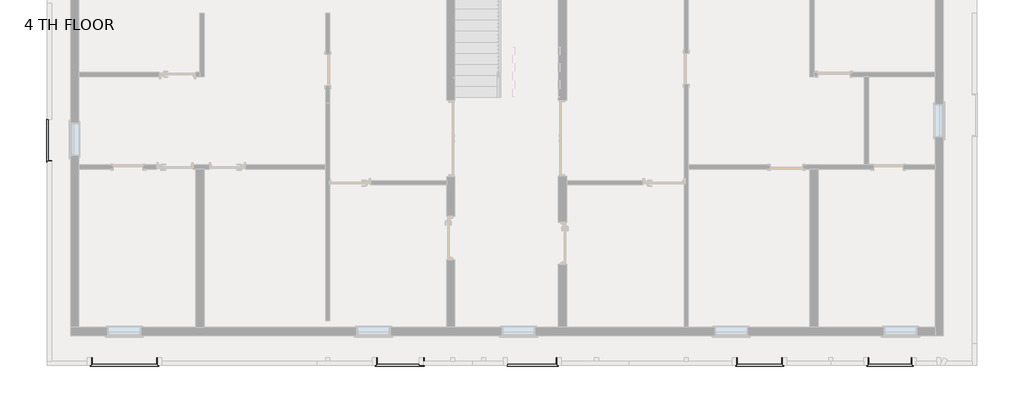
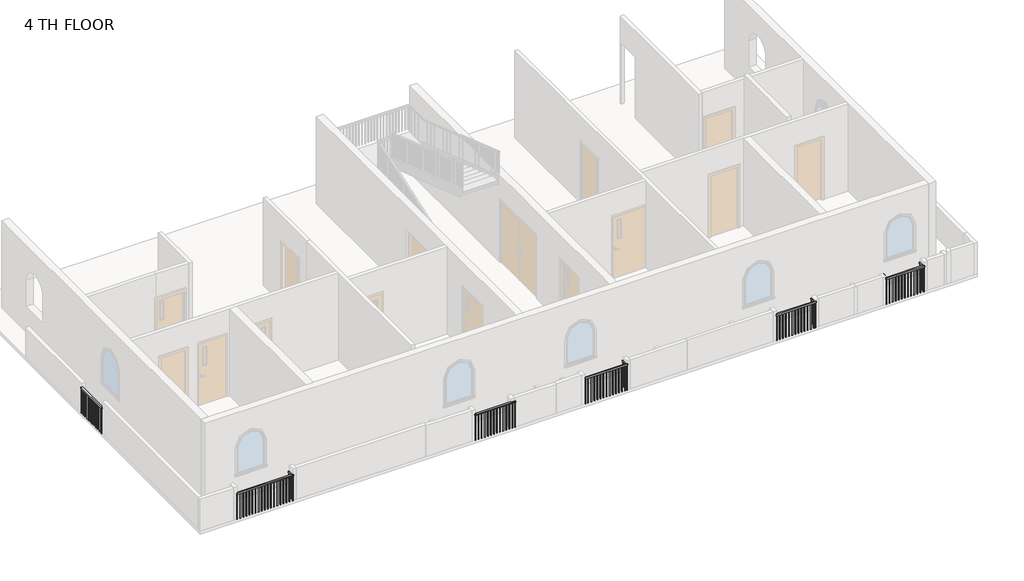
# One storey, part 3 of 7: 6 railings.
"""IFC4 building model written with IfcOpenShell, lengths in millimetres."""

from ifc_helpers import new_model, si_unit, frame, origin, place, context, project, spatial, polyline, outline, extrude, faceted_brep, element, save

model = new_model("IFC4")

# Units and contexts
model_context = context("Model", 3, world=origin())
ifc_project = project(units=[si_unit("LENGTHUNIT", "METRE", prefix="MILLI")], contexts=[model_context])

# Site, building, storey
site = spatial("IfcSite", under=ifc_project)
building = spatial("IfcBuilding", under=site)
storey = spatial("IfcBuildingStorey", under=building, Name="4 TH FLOOR", Elevation=12801.6)

# Railings
placement = place(None, origin())
element("IfcRailing", 1, ObjectType="Handrail - Rectangular", at=placement, inside=storey, context=model_context, shape_type="SolidModel", body=[
    faceted_brep([(-11856.9067989, -4623.6932193, 13716.0), (-11856.9067989, -4623.6932193, 13665.2), (-11907.7067989, -4623.6932193, 13665.2), (-11907.7067989, -4623.6932193, 13716.0), (-11856.9067989, -4801.4932661, 13716.0), (-11856.9067989, -4801.4932661, 13665.2), (-11907.7067989, -4852.2932661, 13665.2), (-11907.7067989, -4852.2932661, 13716.0), (-10071.3470335, -4801.4932661, 13716.0), (-10071.3470335, -4801.4932661, 13665.2), (-10020.5470335, -4852.2932661, 13665.2), (-10020.5470335, -4852.2932661, 13716.0), (-10071.3470335, -4623.6932193, 13716.0), (-10020.5470335, -4623.6932193, 13716.0), (-10020.5470335, -4623.6932193, 13665.2), (-10071.3470335, -4623.6932193, 13665.2)], [[[0, 1, 2, 3]], [[1, 0, 4, 5]], [[2, 1, 5, 6]], [[3, 2, 6, 7]], [[0, 3, 7, 4]], [[5, 4, 8, 9]], [[6, 5, 9, 10]], [[7, 6, 10, 11]], [[4, 7, 11, 8]], [[12, 13, 14, 15]], [[9, 8, 12, 15]], [[10, 9, 15, 14]], [[11, 10, 14, 13]], [[8, 11, 13, 12]]]),
    extrude(outline(polyline([(-10036.4220335, -4633.2182661), (-10055.4720335, -4633.2182661), (-10055.4720335, -4614.1682661), (-10036.4220335, -4614.1682661), (-10036.4220335, -4633.2182661)])), frame((0.0, 0.0, 12801.6), z_axis=(0.0, 0.0, 1.0), x_axis=(1.0, 0.0, 0.0)), (0.0, 0.0, 1.0), 863.6),
    extrude(outline(polyline([(-10036.4220335, -4734.8182661), (-10055.4720335, -4734.8182661), (-10055.4720335, -4715.7682661), (-10036.4220335, -4715.7682661), (-10036.4220335, -4734.8182661)])), frame((0.0, 0.0, 12801.6), z_axis=(0.0, 0.0, 1.0), x_axis=(1.0, 0.0, 0.0)), (0.0, 0.0, 1.0), 863.6),
    extrude(outline(polyline([(-10063.0317989, -4836.4182661), (-10063.0317989, -4817.3682661), (-10043.9817989, -4817.3682661), (-10043.9817989, -4836.4182661), (-10063.0317989, -4836.4182661)])), frame((0.0, 0.0, 12801.6), z_axis=(0.0, 0.0, 1.0), x_axis=(1.0, 0.0, 0.0)), (0.0, 0.0, 1.0), 863.6),
    extrude(outline(polyline([(-10164.6317989, -4836.4182661), (-10164.6317989, -4817.3682661), (-10145.5817989, -4817.3682661), (-10145.5817989, -4836.4182661), (-10164.6317989, -4836.4182661)])), frame((0.0, 0.0, 12801.6), z_axis=(0.0, 0.0, 1.0), x_axis=(1.0, 0.0, 0.0)), (0.0, 0.0, 1.0), 863.6),
    extrude(outline(polyline([(-10266.2317989, -4836.4182661), (-10266.2317989, -4817.3682661), (-10247.1817989, -4817.3682661), (-10247.1817989, -4836.4182661), (-10266.2317989, -4836.4182661)])), frame((0.0, 0.0, 12801.6), z_axis=(0.0, 0.0, 1.0), x_axis=(1.0, 0.0, 0.0)), (0.0, 0.0, 1.0), 863.6),
    extrude(outline(polyline([(-10367.8317989, -4836.4182661), (-10367.8317989, -4817.3682661), (-10348.7817989, -4817.3682661), (-10348.7817989, -4836.4182661), (-10367.8317989, -4836.4182661)])), frame((0.0, 0.0, 12801.6), z_axis=(0.0, 0.0, 1.0), x_axis=(1.0, 0.0, 0.0)), (0.0, 0.0, 1.0), 863.6),
    extrude(outline(polyline([(-10469.4317989, -4836.4182661), (-10469.4317989, -4817.3682661), (-10450.3817989, -4817.3682661), (-10450.3817989, -4836.4182661), (-10469.4317989, -4836.4182661)])), frame((0.0, 0.0, 12801.6), z_axis=(0.0, 0.0, 1.0), x_axis=(1.0, 0.0, 0.0)), (0.0, 0.0, 1.0), 863.6),
    extrude(outline(polyline([(-10571.0317989, -4836.4182661), (-10571.0317989, -4817.3682661), (-10551.9817989, -4817.3682661), (-10551.9817989, -4836.4182661), (-10571.0317989, -4836.4182661)])), frame((0.0, 0.0, 12801.6), z_axis=(0.0, 0.0, 1.0), x_axis=(1.0, 0.0, 0.0)), (0.0, 0.0, 1.0), 863.6),
    extrude(outline(polyline([(-10672.6317989, -4836.4182661), (-10672.6317989, -4817.3682661), (-10653.5817989, -4817.3682661), (-10653.5817989, -4836.4182661), (-10672.6317989, -4836.4182661)])), frame((0.0, 0.0, 12801.6), z_axis=(0.0, 0.0, 1.0), x_axis=(1.0, 0.0, 0.0)), (0.0, 0.0, 1.0), 863.6),
    extrude(outline(polyline([(-10774.2317989, -4836.4182661), (-10774.2317989, -4817.3682661), (-10755.1817989, -4817.3682661), (-10755.1817989, -4836.4182661), (-10774.2317989, -4836.4182661)])), frame((0.0, 0.0, 12801.6), z_axis=(0.0, 0.0, 1.0), x_axis=(1.0, 0.0, 0.0)), (0.0, 0.0, 1.0), 863.6),
    extrude(outline(polyline([(-10875.8317989, -4836.4182661), (-10875.8317989, -4817.3682661), (-10856.7817989, -4817.3682661), (-10856.7817989, -4836.4182661), (-10875.8317989, -4836.4182661)])), frame((0.0, 0.0, 12801.6), z_axis=(0.0, 0.0, 1.0), x_axis=(1.0, 0.0, 0.0)), (0.0, 0.0, 1.0), 863.6),
    extrude(outline(polyline([(-10977.4317989, -4836.4182661), (-10977.4317989, -4817.3682661), (-10958.3817989, -4817.3682661), (-10958.3817989, -4836.4182661), (-10977.4317989, -4836.4182661)])), frame((0.0, 0.0, 12801.6), z_axis=(0.0, 0.0, 1.0), x_axis=(1.0, 0.0, 0.0)), (0.0, 0.0, 1.0), 863.6),
    extrude(outline(polyline([(-11079.0317989, -4836.4182661), (-11079.0317989, -4817.3682661), (-11059.9817989, -4817.3682661), (-11059.9817989, -4836.4182661), (-11079.0317989, -4836.4182661)])), frame((0.0, 0.0, 12801.6), z_axis=(0.0, 0.0, 1.0), x_axis=(1.0, 0.0, 0.0)), (0.0, 0.0, 1.0), 863.6),
    extrude(outline(polyline([(-11180.6317989, -4836.4182661), (-11180.6317989, -4817.3682661), (-11161.5817989, -4817.3682661), (-11161.5817989, -4836.4182661), (-11180.6317989, -4836.4182661)])), frame((0.0, 0.0, 12801.6), z_axis=(0.0, 0.0, 1.0), x_axis=(1.0, 0.0, 0.0)), (0.0, 0.0, 1.0), 863.6),
    extrude(outline(polyline([(-11282.2317989, -4836.4182661), (-11282.2317989, -4817.3682661), (-11263.1817989, -4817.3682661), (-11263.1817989, -4836.4182661), (-11282.2317989, -4836.4182661)])), frame((0.0, 0.0, 12801.6), z_axis=(0.0, 0.0, 1.0), x_axis=(1.0, 0.0, 0.0)), (0.0, 0.0, 1.0), 863.6),
    extrude(outline(polyline([(-11383.8317989, -4836.4182661), (-11383.8317989, -4817.3682661), (-11364.7817989, -4817.3682661), (-11364.7817989, -4836.4182661), (-11383.8317989, -4836.4182661)])), frame((0.0, 0.0, 12801.6), z_axis=(0.0, 0.0, 1.0), x_axis=(1.0, 0.0, 0.0)), (0.0, 0.0, 1.0), 863.6),
    extrude(outline(polyline([(-11485.4317989, -4836.4182661), (-11485.4317989, -4817.3682661), (-11466.3817989, -4817.3682661), (-11466.3817989, -4836.4182661), (-11485.4317989, -4836.4182661)])), frame((0.0, 0.0, 12801.6), z_axis=(0.0, 0.0, 1.0), x_axis=(1.0, 0.0, 0.0)), (0.0, 0.0, 1.0), 863.6),
    extrude(outline(polyline([(-11587.0317989, -4836.4182661), (-11587.0317989, -4817.3682661), (-11567.9817989, -4817.3682661), (-11567.9817989, -4836.4182661), (-11587.0317989, -4836.4182661)])), frame((0.0, 0.0, 12801.6), z_axis=(0.0, 0.0, 1.0), x_axis=(1.0, 0.0, 0.0)), (0.0, 0.0, 1.0), 863.6),
    extrude(outline(polyline([(-11688.6317989, -4836.4182661), (-11688.6317989, -4817.3682661), (-11669.5817989, -4817.3682661), (-11669.5817989, -4836.4182661), (-11688.6317989, -4836.4182661)])), frame((0.0, 0.0, 12801.6), z_axis=(0.0, 0.0, 1.0), x_axis=(1.0, 0.0, 0.0)), (0.0, 0.0, 1.0), 863.6),
    extrude(outline(polyline([(-11790.2317989, -4836.4182661), (-11790.2317989, -4817.3682661), (-11771.1817989, -4817.3682661), (-11771.1817989, -4836.4182661), (-11790.2317989, -4836.4182661)])), frame((0.0, 0.0, 12801.6), z_axis=(0.0, 0.0, 1.0), x_axis=(1.0, 0.0, 0.0)), (0.0, 0.0, 1.0), 863.6),
    extrude(outline(polyline([(-11891.8317989, -4817.3682193), (-11872.7817989, -4817.3682193), (-11872.7817989, -4836.4182193), (-11891.8317989, -4836.4182193), (-11891.8317989, -4817.3682193)])), frame((0.0, 0.0, 12801.6), z_axis=(0.0, 0.0, 1.0), x_axis=(1.0, 0.0, 0.0)), (0.0, 0.0, 1.0), 863.6),
    extrude(outline(polyline([(-11891.8317989, -4715.7682193), (-11872.7817989, -4715.7682193), (-11872.7817989, -4734.8182193), (-11891.8317989, -4734.8182193), (-11891.8317989, -4715.7682193)])), frame((0.0, 0.0, 12801.6), z_axis=(0.0, 0.0, 1.0), x_axis=(1.0, 0.0, 0.0)), (0.0, 0.0, 1.0), 863.6),
    extrude(outline(polyline([(-10055.4720335, -4836.4182661), (-10055.4720335, -4817.3682661), (-10036.4220335, -4817.3682661), (-10036.4220335, -4836.4182661), (-10055.4720335, -4836.4182661)])), frame((0.0, 0.0, 12801.6), z_axis=(0.0, 0.0, 1.0), x_axis=(1.0, 0.0, 0.0)), (0.0, 0.0, 1.0), 863.6),
    extrude(outline(polyline([(-11891.8317989, -4817.3682661), (-11872.7817989, -4817.3682661), (-11872.7817989, -4836.4182661), (-11891.8317989, -4836.4182661), (-11891.8317989, -4817.3682661)])), frame((0.0, 0.0, 12801.6), z_axis=(0.0, 0.0, 1.0), x_axis=(1.0, 0.0, 0.0)), (0.0, 0.0, 1.0), 863.6),
    extrude(outline(polyline([(-10036.4220335, -4642.7432193), (-10055.4720335, -4642.7432193), (-10055.4720335, -4623.6932193), (-10036.4220335, -4623.6932193), (-10036.4220335, -4642.7432193)])), frame((0.0, 0.0, 12801.6), z_axis=(0.0, 0.0, 1.0), x_axis=(1.0, 0.0, 0.0)), (0.0, 0.0, 1.0), 863.6),
    extrude(outline(polyline([(-11891.8317989, -4623.6932193), (-11872.7817989, -4623.6932193), (-11872.7817989, -4642.7432193), (-11891.8317989, -4642.7432193), (-11891.8317989, -4623.6932193)])), frame((0.0, 0.0, 12801.6), z_axis=(0.0, 0.0, 1.0), x_axis=(1.0, 0.0, 0.0)), (0.0, 0.0, 1.0), 863.6),
])
element("IfcRailing", 2, ObjectType="Handrail - Rectangular", at=placement, inside=storey, context=model_context, shape_type="SolidModel", body=[
    faceted_brep([(-3995.0987995, -4623.6932193, 13716.0), (-3995.0987995, -4623.6932193, 13665.2), (-4045.8987995, -4623.6932193, 13665.2), (-4045.8987995, -4623.6932193, 13716.0), (-3995.0987995, -4801.4932661, 13716.0), (-3995.0987995, -4801.4932661, 13665.2), (-4045.8987995, -4852.2932661, 13665.2), (-4045.8987995, -4852.2932661, 13716.0), (-2750.4987995, -4801.4932661, 13716.0), (-2750.4987995, -4801.4932661, 13665.2), (-2699.6987995, -4852.2932661, 13665.2), (-2699.6987995, -4852.2932661, 13716.0), (-2750.4987995, -4623.6932193, 13716.0), (-2699.6987995, -4623.6932193, 13716.0), (-2699.6987995, -4623.6932193, 13665.2), (-2750.4987995, -4623.6932193, 13665.2)], [[[0, 1, 2, 3]], [[1, 0, 4, 5]], [[2, 1, 5, 6]], [[3, 2, 6, 7]], [[0, 3, 7, 4]], [[5, 4, 8, 9]], [[6, 5, 9, 10]], [[7, 6, 10, 11]], [[4, 7, 11, 8]], [[12, 13, 14, 15]], [[9, 8, 12, 15]], [[10, 9, 15, 14]], [[11, 10, 14, 13]], [[8, 11, 13, 12]]]),
    extrude(outline(polyline([(-2715.5737995, -4633.2182661), (-2734.6237995, -4633.2182661), (-2734.6237995, -4614.1682661), (-2715.5737995, -4614.1682661), (-2715.5737995, -4633.2182661)])), frame((0.0, 0.0, 12801.6), z_axis=(0.0, 0.0, 1.0), x_axis=(1.0, 0.0, 0.0)), (0.0, 0.0, 1.0), 863.6),
    extrude(outline(polyline([(-2715.5737995, -4734.8182661), (-2734.6237995, -4734.8182661), (-2734.6237995, -4715.7682661), (-2715.5737995, -4715.7682661), (-2715.5737995, -4734.8182661)])), frame((0.0, 0.0, 12801.6), z_axis=(0.0, 0.0, 1.0), x_axis=(1.0, 0.0, 0.0)), (0.0, 0.0, 1.0), 863.6),
    extrude(outline(polyline([(-2810.8237995, -4836.4182661), (-2810.8237995, -4817.3682661), (-2791.7737995, -4817.3682661), (-2791.7737995, -4836.4182661), (-2810.8237995, -4836.4182661)])), frame((0.0, 0.0, 12801.6), z_axis=(0.0, 0.0, 1.0), x_axis=(1.0, 0.0, 0.0)), (0.0, 0.0, 1.0), 863.6),
    extrude(outline(polyline([(-2912.4237995, -4836.4182661), (-2912.4237995, -4817.3682661), (-2893.3737995, -4817.3682661), (-2893.3737995, -4836.4182661), (-2912.4237995, -4836.4182661)])), frame((0.0, 0.0, 12801.6), z_axis=(0.0, 0.0, 1.0), x_axis=(1.0, 0.0, 0.0)), (0.0, 0.0, 1.0), 863.6),
    extrude(outline(polyline([(-3014.0237995, -4836.4182661), (-3014.0237995, -4817.3682661), (-2994.9737995, -4817.3682661), (-2994.9737995, -4836.4182661), (-3014.0237995, -4836.4182661)])), frame((0.0, 0.0, 12801.6), z_axis=(0.0, 0.0, 1.0), x_axis=(1.0, 0.0, 0.0)), (0.0, 0.0, 1.0), 863.6),
    extrude(outline(polyline([(-3115.6237995, -4836.4182661), (-3115.6237995, -4817.3682661), (-3096.5737995, -4817.3682661), (-3096.5737995, -4836.4182661), (-3115.6237995, -4836.4182661)])), frame((0.0, 0.0, 12801.6), z_axis=(0.0, 0.0, 1.0), x_axis=(1.0, 0.0, 0.0)), (0.0, 0.0, 1.0), 863.6),
    extrude(outline(polyline([(-3217.2237995, -4836.4182661), (-3217.2237995, -4817.3682661), (-3198.1737995, -4817.3682661), (-3198.1737995, -4836.4182661), (-3217.2237995, -4836.4182661)])), frame((0.0, 0.0, 12801.6), z_axis=(0.0, 0.0, 1.0), x_axis=(1.0, 0.0, 0.0)), (0.0, 0.0, 1.0), 863.6),
    extrude(outline(polyline([(-3318.8237995, -4836.4182661), (-3318.8237995, -4817.3682661), (-3299.7737995, -4817.3682661), (-3299.7737995, -4836.4182661), (-3318.8237995, -4836.4182661)])), frame((0.0, 0.0, 12801.6), z_axis=(0.0, 0.0, 1.0), x_axis=(1.0, 0.0, 0.0)), (0.0, 0.0, 1.0), 863.6),
    extrude(outline(polyline([(-3420.4237995, -4836.4182661), (-3420.4237995, -4817.3682661), (-3401.3737995, -4817.3682661), (-3401.3737995, -4836.4182661), (-3420.4237995, -4836.4182661)])), frame((0.0, 0.0, 12801.6), z_axis=(0.0, 0.0, 1.0), x_axis=(1.0, 0.0, 0.0)), (0.0, 0.0, 1.0), 863.6),
    extrude(outline(polyline([(-3522.0237995, -4836.4182661), (-3522.0237995, -4817.3682661), (-3502.9737995, -4817.3682661), (-3502.9737995, -4836.4182661), (-3522.0237995, -4836.4182661)])), frame((0.0, 0.0, 12801.6), z_axis=(0.0, 0.0, 1.0), x_axis=(1.0, 0.0, 0.0)), (0.0, 0.0, 1.0), 863.6),
    extrude(outline(polyline([(-3623.6237995, -4836.4182661), (-3623.6237995, -4817.3682661), (-3604.5737995, -4817.3682661), (-3604.5737995, -4836.4182661), (-3623.6237995, -4836.4182661)])), frame((0.0, 0.0, 12801.6), z_axis=(0.0, 0.0, 1.0), x_axis=(1.0, 0.0, 0.0)), (0.0, 0.0, 1.0), 863.6),
    extrude(outline(polyline([(-3725.2237995, -4836.4182661), (-3725.2237995, -4817.3682661), (-3706.1737995, -4817.3682661), (-3706.1737995, -4836.4182661), (-3725.2237995, -4836.4182661)])), frame((0.0, 0.0, 12801.6), z_axis=(0.0, 0.0, 1.0), x_axis=(1.0, 0.0, 0.0)), (0.0, 0.0, 1.0), 863.6),
    extrude(outline(polyline([(-3826.8237995, -4836.4182661), (-3826.8237995, -4817.3682661), (-3807.7737995, -4817.3682661), (-3807.7737995, -4836.4182661), (-3826.8237995, -4836.4182661)])), frame((0.0, 0.0, 12801.6), z_axis=(0.0, 0.0, 1.0), x_axis=(1.0, 0.0, 0.0)), (0.0, 0.0, 1.0), 863.6),
    extrude(outline(polyline([(-3928.4237995, -4836.4182661), (-3928.4237995, -4817.3682661), (-3909.3737995, -4817.3682661), (-3909.3737995, -4836.4182661), (-3928.4237995, -4836.4182661)])), frame((0.0, 0.0, 12801.6), z_axis=(0.0, 0.0, 1.0), x_axis=(1.0, 0.0, 0.0)), (0.0, 0.0, 1.0), 863.6),
    extrude(outline(polyline([(-4030.0237995, -4817.3682193), (-4010.9737995, -4817.3682193), (-4010.9737995, -4836.4182193), (-4030.0237995, -4836.4182193), (-4030.0237995, -4817.3682193)])), frame((0.0, 0.0, 12801.6), z_axis=(0.0, 0.0, 1.0), x_axis=(1.0, 0.0, 0.0)), (0.0, 0.0, 1.0), 863.6),
    extrude(outline(polyline([(-4030.0237995, -4715.7682193), (-4010.9737995, -4715.7682193), (-4010.9737995, -4734.8182193), (-4030.0237995, -4734.8182193), (-4030.0237995, -4715.7682193)])), frame((0.0, 0.0, 12801.6), z_axis=(0.0, 0.0, 1.0), x_axis=(1.0, 0.0, 0.0)), (0.0, 0.0, 1.0), 863.6),
    extrude(outline(polyline([(-2734.6237995, -4836.4182661), (-2734.6237995, -4817.3682661), (-2715.5737995, -4817.3682661), (-2715.5737995, -4836.4182661), (-2734.6237995, -4836.4182661)])), frame((0.0, 0.0, 12801.6), z_axis=(0.0, 0.0, 1.0), x_axis=(1.0, 0.0, 0.0)), (0.0, 0.0, 1.0), 863.6),
    extrude(outline(polyline([(-4030.0237995, -4817.3682661), (-4010.9737995, -4817.3682661), (-4010.9737995, -4836.4182661), (-4030.0237995, -4836.4182661), (-4030.0237995, -4817.3682661)])), frame((0.0, 0.0, 12801.6), z_axis=(0.0, 0.0, 1.0), x_axis=(1.0, 0.0, 0.0)), (0.0, 0.0, 1.0), 863.6),
    extrude(outline(polyline([(-2715.5737995, -4642.7432193), (-2734.6237995, -4642.7432193), (-2734.6237995, -4623.6932193), (-2715.5737995, -4623.6932193), (-2715.5737995, -4642.7432193)])), frame((0.0, 0.0, 12801.6), z_axis=(0.0, 0.0, 1.0), x_axis=(1.0, 0.0, 0.0)), (0.0, 0.0, 1.0), 863.6),
    extrude(outline(polyline([(-4030.0237995, -4623.6932193), (-4010.9737995, -4623.6932193), (-4010.9737995, -4642.7432193), (-4030.0237995, -4642.7432193), (-4030.0237995, -4623.6932193)])), frame((0.0, 0.0, 12801.6), z_axis=(0.0, 0.0, 1.0), x_axis=(1.0, 0.0, 0.0)), (0.0, 0.0, 1.0), 863.6),
])
element("IfcRailing", 3, ObjectType="Handrail - Rectangular", at=placement, inside=storey, context=model_context, shape_type="SolidModel", body=[
    faceted_brep([(-406.2065315, -4801.4932661, 13716.0), (-406.2065315, -4801.4932661, 13665.2), (-406.2065315, -4852.2932661, 13665.2), (-406.2065315, -4852.2932661, 13716.0), (944.6932011, -4801.4932661, 13716.0), (944.6932011, -4801.4932661, 13665.2), (995.4932011, -4852.2932661, 13665.2), (995.4932011, -4852.2932661, 13716.0), (944.6932011, -4623.6932193, 13716.0), (995.4932011, -4623.6932193, 13716.0), (995.4932011, -4623.6932193, 13665.2), (944.6932011, -4623.6932193, 13665.2)], [[[0, 1, 2, 3]], [[1, 0, 4, 5]], [[2, 1, 5, 6]], [[3, 2, 6, 7]], [[0, 3, 7, 4]], [[8, 9, 10, 11]], [[5, 4, 8, 11]], [[6, 5, 11, 10]], [[7, 6, 10, 9]], [[4, 7, 9, 8]]]),
    extrude(outline(polyline([(979.6182011, -4633.2182661), (960.5682011, -4633.2182661), (960.5682011, -4614.1682661), (979.6182011, -4614.1682661), (979.6182011, -4633.2182661)])), frame((0.0, 0.0, 12801.6), z_axis=(0.0, 0.0, 1.0), x_axis=(1.0, 0.0, 0.0)), (0.0, 0.0, 1.0), 863.6),
    extrude(outline(polyline([(979.6182011, -4734.8182661), (960.5682011, -4734.8182661), (960.5682011, -4715.7682661), (979.6182011, -4715.7682661), (979.6182011, -4734.8182661)])), frame((0.0, 0.0, 12801.6), z_axis=(0.0, 0.0, 1.0), x_axis=(1.0, 0.0, 0.0)), (0.0, 0.0, 1.0), 863.6),
    extrude(outline(polyline([(905.0684685, -4836.4182661), (905.0684685, -4817.3682661), (924.1184685, -4817.3682661), (924.1184685, -4836.4182661), (905.0684685, -4836.4182661)])), frame((0.0, 0.0, 12801.6), z_axis=(0.0, 0.0, 1.0), x_axis=(1.0, 0.0, 0.0)), (0.0, 0.0, 1.0), 863.6),
    extrude(outline(polyline([(803.4684685, -4836.4182661), (803.4684685, -4817.3682661), (822.5184685, -4817.3682661), (822.5184685, -4836.4182661), (803.4684685, -4836.4182661)])), frame((0.0, 0.0, 12801.6), z_axis=(0.0, 0.0, 1.0), x_axis=(1.0, 0.0, 0.0)), (0.0, 0.0, 1.0), 863.6),
    extrude(outline(polyline([(701.8684685, -4836.4182661), (701.8684685, -4817.3682661), (720.9184685, -4817.3682661), (720.9184685, -4836.4182661), (701.8684685, -4836.4182661)])), frame((0.0, 0.0, 12801.6), z_axis=(0.0, 0.0, 1.0), x_axis=(1.0, 0.0, 0.0)), (0.0, 0.0, 1.0), 863.6),
    extrude(outline(polyline([(600.2684685, -4836.4182661), (600.2684685, -4817.3682661), (619.3184685, -4817.3682661), (619.3184685, -4836.4182661), (600.2684685, -4836.4182661)])), frame((0.0, 0.0, 12801.6), z_axis=(0.0, 0.0, 1.0), x_axis=(1.0, 0.0, 0.0)), (0.0, 0.0, 1.0), 863.6),
    extrude(outline(polyline([(498.6684685, -4836.4182661), (498.6684685, -4817.3682661), (517.7184685, -4817.3682661), (517.7184685, -4836.4182661), (498.6684685, -4836.4182661)])), frame((0.0, 0.0, 12801.6), z_axis=(0.0, 0.0, 1.0), x_axis=(1.0, 0.0, 0.0)), (0.0, 0.0, 1.0), 863.6),
    extrude(outline(polyline([(397.0684685, -4836.4182661), (397.0684685, -4817.3682661), (416.1184685, -4817.3682661), (416.1184685, -4836.4182661), (397.0684685, -4836.4182661)])), frame((0.0, 0.0, 12801.6), z_axis=(0.0, 0.0, 1.0), x_axis=(1.0, 0.0, 0.0)), (0.0, 0.0, 1.0), 863.6),
    extrude(outline(polyline([(295.4684685, -4836.4182661), (295.4684685, -4817.3682661), (314.5184685, -4817.3682661), (314.5184685, -4836.4182661), (295.4684685, -4836.4182661)])), frame((0.0, 0.0, 12801.6), z_axis=(0.0, 0.0, 1.0), x_axis=(1.0, 0.0, 0.0)), (0.0, 0.0, 1.0), 863.6),
    extrude(outline(polyline([(193.8684685, -4836.4182661), (193.8684685, -4817.3682661), (212.9184685, -4817.3682661), (212.9184685, -4836.4182661), (193.8684685, -4836.4182661)])), frame((0.0, 0.0, 12801.6), z_axis=(0.0, 0.0, 1.0), x_axis=(1.0, 0.0, 0.0)), (0.0, 0.0, 1.0), 863.6),
    extrude(outline(polyline([(92.2684685, -4836.4182661), (92.2684685, -4817.3682661), (111.3184685, -4817.3682661), (111.3184685, -4836.4182661), (92.2684685, -4836.4182661)])), frame((0.0, 0.0, 12801.6), z_axis=(0.0, 0.0, 1.0), x_axis=(1.0, 0.0, 0.0)), (0.0, 0.0, 1.0), 863.6),
    extrude(outline(polyline([(-9.3315315, -4836.4182661), (-9.3315315, -4817.3682661), (9.7184685, -4817.3682661), (9.7184685, -4836.4182661), (-9.3315315, -4836.4182661)])), frame((0.0, 0.0, 12801.6), z_axis=(0.0, 0.0, 1.0), x_axis=(1.0, 0.0, 0.0)), (0.0, 0.0, 1.0), 863.6),
    extrude(outline(polyline([(-110.9315315, -4836.4182661), (-110.9315315, -4817.3682661), (-91.8815315, -4817.3682661), (-91.8815315, -4836.4182661), (-110.9315315, -4836.4182661)])), frame((0.0, 0.0, 12801.6), z_axis=(0.0, 0.0, 1.0), x_axis=(1.0, 0.0, 0.0)), (0.0, 0.0, 1.0), 863.6),
    extrude(outline(polyline([(-212.5315315, -4836.4182661), (-212.5315315, -4817.3682661), (-193.4815315, -4817.3682661), (-193.4815315, -4836.4182661), (-212.5315315, -4836.4182661)])), frame((0.0, 0.0, 12801.6), z_axis=(0.0, 0.0, 1.0), x_axis=(1.0, 0.0, 0.0)), (0.0, 0.0, 1.0), 863.6),
    extrude(outline(polyline([(-314.1315315, -4836.4182661), (-314.1315315, -4817.3682661), (-295.0815315, -4817.3682661), (-295.0815315, -4836.4182661), (-314.1315315, -4836.4182661)])), frame((0.0, 0.0, 12801.6), z_axis=(0.0, 0.0, 1.0), x_axis=(1.0, 0.0, 0.0)), (0.0, 0.0, 1.0), 863.6),
    extrude(outline(polyline([(960.5682011, -4836.4182661), (960.5682011, -4817.3682661), (979.6182011, -4817.3682661), (979.6182011, -4836.4182661), (960.5682011, -4836.4182661)])), frame((0.0, 0.0, 12801.6), z_axis=(0.0, 0.0, 1.0), x_axis=(1.0, 0.0, 0.0)), (0.0, 0.0, 1.0), 863.6),
    extrude(outline(polyline([(979.6182011, -4642.7432193), (960.5682011, -4642.7432193), (960.5682011, -4623.6932193), (979.6182011, -4623.6932193), (979.6182011, -4642.7432193)])), frame((0.0, 0.0, 12801.6), z_axis=(0.0, 0.0, 1.0), x_axis=(1.0, 0.0, 0.0)), (0.0, 0.0, 1.0), 863.6),
    extrude(outline(polyline([(-406.2065315, -4836.4182661), (-406.2065315, -4817.3682661), (-387.1565315, -4817.3682661), (-387.1565315, -4836.4182661), (-406.2065315, -4836.4182661)])), frame((0.0, 0.0, 12801.6), z_axis=(0.0, 0.0, 1.0), x_axis=(1.0, 0.0, 0.0)), (0.0, 0.0, 1.0), 863.6),
])
element("IfcRailing", 4, ObjectType="Handrail - Rectangular", at=placement, inside=storey, context=model_context, shape_type="SolidModel", body=[
    faceted_brep([(5942.6512082, -4623.6932193, 13716.0), (5942.6512082, -4623.6932193, 13665.2), (5891.8512082, -4623.6932193, 13665.2), (5891.8512082, -4623.6932193, 13716.0), (5942.6512082, -4801.4932661, 13716.0), (5942.6512082, -4801.4932661, 13665.2), (5891.8512082, -4852.2932661, 13665.2), (5891.8512082, -4852.2932661, 13716.0), (7164.9011643, -4801.4932661, 13716.0), (7164.9011643, -4801.4932661, 13665.2), (7215.7011643, -4852.2932661, 13665.2), (7215.7011643, -4852.2932661, 13716.0), (7164.9011643, -4623.6932193, 13716.0), (7215.7011643, -4623.6932193, 13716.0), (7215.7011643, -4623.6932193, 13665.2), (7164.9011643, -4623.6932193, 13665.2)], [[[0, 1, 2, 3]], [[1, 0, 4, 5]], [[2, 1, 5, 6]], [[3, 2, 6, 7]], [[0, 3, 7, 4]], [[5, 4, 8, 9]], [[6, 5, 9, 10]], [[7, 6, 10, 11]], [[4, 7, 11, 8]], [[12, 13, 14, 15]], [[9, 8, 12, 15]], [[10, 9, 15, 14]], [[11, 10, 14, 13]], [[8, 11, 13, 12]]]),
    extrude(outline(polyline([(7199.8261643, -4633.2182661), (7180.7761643, -4633.2182661), (7180.7761643, -4614.1682661), (7199.8261643, -4614.1682661), (7199.8261643, -4633.2182661)])), frame((0.0, 0.0, 12801.6), z_axis=(0.0, 0.0, 1.0), x_axis=(1.0, 0.0, 0.0)), (0.0, 0.0, 1.0), 863.6),
    extrude(outline(polyline([(7199.8261643, -4734.8182661), (7180.7761643, -4734.8182661), (7180.7761643, -4715.7682661), (7199.8261643, -4715.7682661), (7199.8261643, -4734.8182661)])), frame((0.0, 0.0, 12801.6), z_axis=(0.0, 0.0, 1.0), x_axis=(1.0, 0.0, 0.0)), (0.0, 0.0, 1.0), 863.6),
    extrude(outline(polyline([(7126.9262082, -4836.4182661), (7126.9262082, -4817.3682661), (7145.9762082, -4817.3682661), (7145.9762082, -4836.4182661), (7126.9262082, -4836.4182661)])), frame((0.0, 0.0, 12801.6), z_axis=(0.0, 0.0, 1.0), x_axis=(1.0, 0.0, 0.0)), (0.0, 0.0, 1.0), 863.6),
    extrude(outline(polyline([(7025.3262082, -4836.4182661), (7025.3262082, -4817.3682661), (7044.3762082, -4817.3682661), (7044.3762082, -4836.4182661), (7025.3262082, -4836.4182661)])), frame((0.0, 0.0, 12801.6), z_axis=(0.0, 0.0, 1.0), x_axis=(1.0, 0.0, 0.0)), (0.0, 0.0, 1.0), 863.6),
    extrude(outline(polyline([(6923.7262082, -4836.4182661), (6923.7262082, -4817.3682661), (6942.7762082, -4817.3682661), (6942.7762082, -4836.4182661), (6923.7262082, -4836.4182661)])), frame((0.0, 0.0, 12801.6), z_axis=(0.0, 0.0, 1.0), x_axis=(1.0, 0.0, 0.0)), (0.0, 0.0, 1.0), 863.6),
    extrude(outline(polyline([(6822.1262082, -4836.4182661), (6822.1262082, -4817.3682661), (6841.1762082, -4817.3682661), (6841.1762082, -4836.4182661), (6822.1262082, -4836.4182661)])), frame((0.0, 0.0, 12801.6), z_axis=(0.0, 0.0, 1.0), x_axis=(1.0, 0.0, 0.0)), (0.0, 0.0, 1.0), 863.6),
    extrude(outline(polyline([(6720.5262082, -4836.4182661), (6720.5262082, -4817.3682661), (6739.5762082, -4817.3682661), (6739.5762082, -4836.4182661), (6720.5262082, -4836.4182661)])), frame((0.0, 0.0, 12801.6), z_axis=(0.0, 0.0, 1.0), x_axis=(1.0, 0.0, 0.0)), (0.0, 0.0, 1.0), 863.6),
    extrude(outline(polyline([(6618.9262082, -4836.4182661), (6618.9262082, -4817.3682661), (6637.9762082, -4817.3682661), (6637.9762082, -4836.4182661), (6618.9262082, -4836.4182661)])), frame((0.0, 0.0, 12801.6), z_axis=(0.0, 0.0, 1.0), x_axis=(1.0, 0.0, 0.0)), (0.0, 0.0, 1.0), 863.6),
    extrude(outline(polyline([(6517.3262082, -4836.4182661), (6517.3262082, -4817.3682661), (6536.3762082, -4817.3682661), (6536.3762082, -4836.4182661), (6517.3262082, -4836.4182661)])), frame((0.0, 0.0, 12801.6), z_axis=(0.0, 0.0, 1.0), x_axis=(1.0, 0.0, 0.0)), (0.0, 0.0, 1.0), 863.6),
    extrude(outline(polyline([(6415.7262082, -4836.4182661), (6415.7262082, -4817.3682661), (6434.7762082, -4817.3682661), (6434.7762082, -4836.4182661), (6415.7262082, -4836.4182661)])), frame((0.0, 0.0, 12801.6), z_axis=(0.0, 0.0, 1.0), x_axis=(1.0, 0.0, 0.0)), (0.0, 0.0, 1.0), 863.6),
    extrude(outline(polyline([(6314.1262082, -4836.4182661), (6314.1262082, -4817.3682661), (6333.1762082, -4817.3682661), (6333.1762082, -4836.4182661), (6314.1262082, -4836.4182661)])), frame((0.0, 0.0, 12801.6), z_axis=(0.0, 0.0, 1.0), x_axis=(1.0, 0.0, 0.0)), (0.0, 0.0, 1.0), 863.6),
    extrude(outline(polyline([(6212.5262082, -4836.4182661), (6212.5262082, -4817.3682661), (6231.5762082, -4817.3682661), (6231.5762082, -4836.4182661), (6212.5262082, -4836.4182661)])), frame((0.0, 0.0, 12801.6), z_axis=(0.0, 0.0, 1.0), x_axis=(1.0, 0.0, 0.0)), (0.0, 0.0, 1.0), 863.6),
    extrude(outline(polyline([(6110.9262082, -4836.4182661), (6110.9262082, -4817.3682661), (6129.9762082, -4817.3682661), (6129.9762082, -4836.4182661), (6110.9262082, -4836.4182661)])), frame((0.0, 0.0, 12801.6), z_axis=(0.0, 0.0, 1.0), x_axis=(1.0, 0.0, 0.0)), (0.0, 0.0, 1.0), 863.6),
    extrude(outline(polyline([(6009.3262082, -4836.4182661), (6009.3262082, -4817.3682661), (6028.3762082, -4817.3682661), (6028.3762082, -4836.4182661), (6009.3262082, -4836.4182661)])), frame((0.0, 0.0, 12801.6), z_axis=(0.0, 0.0, 1.0), x_axis=(1.0, 0.0, 0.0)), (0.0, 0.0, 1.0), 863.6),
    extrude(outline(polyline([(5907.7262082, -4817.3682193), (5926.7762082, -4817.3682193), (5926.7762082, -4836.4182193), (5907.7262082, -4836.4182193), (5907.7262082, -4817.3682193)])), frame((0.0, 0.0, 12801.6), z_axis=(0.0, 0.0, 1.0), x_axis=(1.0, 0.0, 0.0)), (0.0, 0.0, 1.0), 863.6),
    extrude(outline(polyline([(5907.7262082, -4715.7682193), (5926.7762082, -4715.7682193), (5926.7762082, -4734.8182193), (5907.7262082, -4734.8182193), (5907.7262082, -4715.7682193)])), frame((0.0, 0.0, 12801.6), z_axis=(0.0, 0.0, 1.0), x_axis=(1.0, 0.0, 0.0)), (0.0, 0.0, 1.0), 863.6),
    extrude(outline(polyline([(7180.7761643, -4836.4182661), (7180.7761643, -4817.3682661), (7199.8261643, -4817.3682661), (7199.8261643, -4836.4182661), (7180.7761643, -4836.4182661)])), frame((0.0, 0.0, 12801.6), z_axis=(0.0, 0.0, 1.0), x_axis=(1.0, 0.0, 0.0)), (0.0, 0.0, 1.0), 863.6),
    extrude(outline(polyline([(5907.7262082, -4817.3682661), (5926.7762082, -4817.3682661), (5926.7762082, -4836.4182661), (5907.7262082, -4836.4182661), (5907.7262082, -4817.3682661)])), frame((0.0, 0.0, 12801.6), z_axis=(0.0, 0.0, 1.0), x_axis=(1.0, 0.0, 0.0)), (0.0, 0.0, 1.0), 863.6),
    extrude(outline(polyline([(7199.8261643, -4642.7432193), (7180.7761643, -4642.7432193), (7180.7761643, -4623.6932193), (7199.8261643, -4623.6932193), (7199.8261643, -4642.7432193)])), frame((0.0, 0.0, 12801.6), z_axis=(0.0, 0.0, 1.0), x_axis=(1.0, 0.0, 0.0)), (0.0, 0.0, 1.0), 863.6),
    extrude(outline(polyline([(5907.7262082, -4623.6932193), (5926.7762082, -4623.6932193), (5926.7762082, -4642.7432193), (5907.7262082, -4642.7432193), (5907.7262082, -4623.6932193)])), frame((0.0, 0.0, 12801.6), z_axis=(0.0, 0.0, 1.0), x_axis=(1.0, 0.0, 0.0)), (0.0, 0.0, 1.0), 863.6),
])
element("IfcRailing", 5, ObjectType="Handrail - Rectangular", at=placement, inside=storey, context=model_context, shape_type="SolidModel", body=[
    faceted_brep([(9562.1512082, -4623.6932193, 13716.0), (9562.1512082, -4623.6932193, 13665.2), (9511.3512082, -4623.6932193, 13665.2), (9511.3512082, -4623.6932193, 13716.0), (9562.1512082, -4801.4932661, 13716.0), (9562.1512082, -4801.4932661, 13665.2), (9511.3512082, -4852.2932661, 13665.2), (9511.3512082, -4852.2932661, 13716.0), (10738.7617205, -4801.4932661, 13716.0), (10738.7617205, -4801.4932661, 13665.2), (10789.5617205, -4852.2932661, 13665.2), (10789.5617205, -4852.2932661, 13716.0), (10738.7617205, -4623.6932193, 13716.0), (10789.5617205, -4623.6932193, 13716.0), (10789.5617205, -4623.6932193, 13665.2), (10738.7617205, -4623.6932193, 13665.2)], [[[0, 1, 2, 3]], [[1, 0, 4, 5]], [[2, 1, 5, 6]], [[3, 2, 6, 7]], [[0, 3, 7, 4]], [[5, 4, 8, 9]], [[6, 5, 9, 10]], [[7, 6, 10, 11]], [[4, 7, 11, 8]], [[12, 13, 14, 15]], [[9, 8, 12, 15]], [[10, 9, 15, 14]], [[11, 10, 14, 13]], [[8, 11, 13, 12]]]),
    extrude(outline(polyline([(10754.6367205, -4633.2182661), (10754.6367205, -4614.1682661), (10773.6867205, -4614.1682661), (10773.6867205, -4633.2182661), (10754.6367205, -4633.2182661)])), frame((0.0, 0.0, 12801.6), z_axis=(0.0, 0.0, 1.0), x_axis=(1.0, 0.0, 0.0)), (0.0, 0.0, 1.0), 863.6),
    extrude(outline(polyline([(10754.6367205, -4734.8182661), (10754.6367205, -4715.7682661), (10773.6867205, -4715.7682661), (10773.6867205, -4734.8182661), (10754.6367205, -4734.8182661)])), frame((0.0, 0.0, 12801.6), z_axis=(0.0, 0.0, 1.0), x_axis=(1.0, 0.0, 0.0)), (0.0, 0.0, 1.0), 863.6),
    extrude(outline(polyline([(10746.4262082, -4817.3682661), (10765.4762082, -4817.3682661), (10765.4762082, -4836.4182661), (10746.4262082, -4836.4182661), (10746.4262082, -4817.3682661)])), frame((0.0, 0.0, 12801.6), z_axis=(0.0, 0.0, 1.0), x_axis=(1.0, 0.0, 0.0)), (0.0, 0.0, 1.0), 863.6),
    extrude(outline(polyline([(10644.8262082, -4817.3682661), (10663.8762082, -4817.3682661), (10663.8762082, -4836.4182661), (10644.8262082, -4836.4182661), (10644.8262082, -4817.3682661)])), frame((0.0, 0.0, 12801.6), z_axis=(0.0, 0.0, 1.0), x_axis=(1.0, 0.0, 0.0)), (0.0, 0.0, 1.0), 863.6),
    extrude(outline(polyline([(10543.2262082, -4817.3682661), (10562.2762082, -4817.3682661), (10562.2762082, -4836.4182661), (10543.2262082, -4836.4182661), (10543.2262082, -4817.3682661)])), frame((0.0, 0.0, 12801.6), z_axis=(0.0, 0.0, 1.0), x_axis=(1.0, 0.0, 0.0)), (0.0, 0.0, 1.0), 863.6),
    extrude(outline(polyline([(10441.6262082, -4817.3682661), (10460.6762082, -4817.3682661), (10460.6762082, -4836.4182661), (10441.6262082, -4836.4182661), (10441.6262082, -4817.3682661)])), frame((0.0, 0.0, 12801.6), z_axis=(0.0, 0.0, 1.0), x_axis=(1.0, 0.0, 0.0)), (0.0, 0.0, 1.0), 863.6),
    extrude(outline(polyline([(10340.0262082, -4817.3682661), (10359.0762082, -4817.3682661), (10359.0762082, -4836.4182661), (10340.0262082, -4836.4182661), (10340.0262082, -4817.3682661)])), frame((0.0, 0.0, 12801.6), z_axis=(0.0, 0.0, 1.0), x_axis=(1.0, 0.0, 0.0)), (0.0, 0.0, 1.0), 863.6),
    extrude(outline(polyline([(10238.4262082, -4817.3682661), (10257.4762082, -4817.3682661), (10257.4762082, -4836.4182661), (10238.4262082, -4836.4182661), (10238.4262082, -4817.3682661)])), frame((0.0, 0.0, 12801.6), z_axis=(0.0, 0.0, 1.0), x_axis=(1.0, 0.0, 0.0)), (0.0, 0.0, 1.0), 863.6),
    extrude(outline(polyline([(10136.8262082, -4817.3682661), (10155.8762082, -4817.3682661), (10155.8762082, -4836.4182661), (10136.8262082, -4836.4182661), (10136.8262082, -4817.3682661)])), frame((0.0, 0.0, 12801.6), z_axis=(0.0, 0.0, 1.0), x_axis=(1.0, 0.0, 0.0)), (0.0, 0.0, 1.0), 863.6),
    extrude(outline(polyline([(10035.2262082, -4817.3682661), (10054.2762082, -4817.3682661), (10054.2762082, -4836.4182661), (10035.2262082, -4836.4182661), (10035.2262082, -4817.3682661)])), frame((0.0, 0.0, 12801.6), z_axis=(0.0, 0.0, 1.0), x_axis=(1.0, 0.0, 0.0)), (0.0, 0.0, 1.0), 863.6),
    extrude(outline(polyline([(9933.6262082, -4817.3682661), (9952.6762082, -4817.3682661), (9952.6762082, -4836.4182661), (9933.6262082, -4836.4182661), (9933.6262082, -4817.3682661)])), frame((0.0, 0.0, 12801.6), z_axis=(0.0, 0.0, 1.0), x_axis=(1.0, 0.0, 0.0)), (0.0, 0.0, 1.0), 863.6),
    extrude(outline(polyline([(9832.0262082, -4817.3682661), (9851.0762082, -4817.3682661), (9851.0762082, -4836.4182661), (9832.0262082, -4836.4182661), (9832.0262082, -4817.3682661)])), frame((0.0, 0.0, 12801.6), z_axis=(0.0, 0.0, 1.0), x_axis=(1.0, 0.0, 0.0)), (0.0, 0.0, 1.0), 863.6),
    extrude(outline(polyline([(9730.4262082, -4817.3682661), (9749.4762082, -4817.3682661), (9749.4762082, -4836.4182661), (9730.4262082, -4836.4182661), (9730.4262082, -4817.3682661)])), frame((0.0, 0.0, 12801.6), z_axis=(0.0, 0.0, 1.0), x_axis=(1.0, 0.0, 0.0)), (0.0, 0.0, 1.0), 863.6),
    extrude(outline(polyline([(9628.8262082, -4817.3682661), (9647.8762082, -4817.3682661), (9647.8762082, -4836.4182661), (9628.8262082, -4836.4182661), (9628.8262082, -4817.3682661)])), frame((0.0, 0.0, 12801.6), z_axis=(0.0, 0.0, 1.0), x_axis=(1.0, 0.0, 0.0)), (0.0, 0.0, 1.0), 863.6),
    extrude(outline(polyline([(9546.2762082, -4817.3682193), (9546.2762082, -4836.4182193), (9527.2262082, -4836.4182193), (9527.2262082, -4817.3682193), (9546.2762082, -4817.3682193)])), frame((0.0, 0.0, 12801.6), z_axis=(0.0, 0.0, 1.0), x_axis=(1.0, 0.0, 0.0)), (0.0, 0.0, 1.0), 863.6),
    extrude(outline(polyline([(9546.2762082, -4715.7682193), (9546.2762082, -4734.8182193), (9527.2262082, -4734.8182193), (9527.2262082, -4715.7682193), (9546.2762082, -4715.7682193)])), frame((0.0, 0.0, 12801.6), z_axis=(0.0, 0.0, 1.0), x_axis=(1.0, 0.0, 0.0)), (0.0, 0.0, 1.0), 863.6),
    extrude(outline(polyline([(10754.6367205, -4817.3682661), (10773.6867205, -4817.3682661), (10773.6867205, -4836.4182661), (10754.6367205, -4836.4182661), (10754.6367205, -4817.3682661)])), frame((0.0, 0.0, 12801.6), z_axis=(0.0, 0.0, 1.0), x_axis=(1.0, 0.0, 0.0)), (0.0, 0.0, 1.0), 863.6),
    extrude(outline(polyline([(9546.2762082, -4817.3682661), (9546.2762082, -4836.4182661), (9527.2262082, -4836.4182661), (9527.2262082, -4817.3682661), (9546.2762082, -4817.3682661)])), frame((0.0, 0.0, 12801.6), z_axis=(0.0, 0.0, 1.0), x_axis=(1.0, 0.0, 0.0)), (0.0, 0.0, 1.0), 863.6),
    extrude(outline(polyline([(10754.6367205, -4642.7432193), (10754.6367205, -4623.6932193), (10773.6867205, -4623.6932193), (10773.6867205, -4642.7432193), (10754.6367205, -4642.7432193)])), frame((0.0, 0.0, 12801.6), z_axis=(0.0, 0.0, 1.0), x_axis=(1.0, 0.0, 0.0)), (0.0, 0.0, 1.0), 863.6),
    extrude(outline(polyline([(9546.2762082, -4623.6932193), (9546.2762082, -4642.7432193), (9527.2262082, -4642.7432193), (9527.2262082, -4623.6932193), (9546.2762082, -4623.6932193)])), frame((0.0, 0.0, 12801.6), z_axis=(0.0, 0.0, 1.0), x_axis=(1.0, 0.0, 0.0)), (0.0, 0.0, 1.0), 863.6),
])
element("IfcRailing", 6, ObjectType="Handrail - Rectangular", at=placement, inside=storey, context=model_context, shape_type="SolidModel", body=[
    faceted_brep([(-13063.4067989, 1953.9604213, 13716.0), (-13063.4067989, 1953.9604213, 13665.2), (-13114.2067989, 1953.9604213, 13665.2), (-13114.2067989, 1953.9604213, 13716.0), (-13063.4067989, 818.2567339, 13716.0), (-13063.4067989, 818.2567339, 13665.2), (-13114.2067989, 767.4567339, 13665.2), (-13114.2067989, 767.4567339, 13716.0), (-12974.5067989, 818.2567339, 13716.0), (-12974.5067989, 767.4567339, 13716.0), (-12974.5067989, 767.4567339, 13665.2), (-12974.5067989, 818.2567339, 13665.2)], [[[0, 1, 2, 3]], [[1, 0, 4, 5]], [[2, 1, 5, 6]], [[3, 2, 6, 7]], [[0, 3, 7, 4]], [[8, 9, 10, 11]], [[5, 4, 8, 11]], [[6, 5, 11, 10]], [[7, 6, 10, 9]], [[4, 7, 9, 8]]]),
    extrude(outline(polyline([(-12996.7317989, 783.3317339), (-12996.7317989, 802.3817339), (-12977.6817989, 802.3817339), (-12977.6817989, 783.3317339), (-12996.7317989, 783.3317339)])), frame((0.0, 0.0, 12801.6), z_axis=(0.0, 0.0, 1.0), x_axis=(1.0, 0.0, 0.0)), (0.0, 0.0, 1.0), 863.6),
    extrude(outline(polyline([(-13098.3317989, 845.8854213), (-13079.2817989, 845.8854213), (-13079.2817989, 826.8354213), (-13098.3317989, 826.8354213), (-13098.3317989, 845.8854213)])), frame((0.0, 0.0, 12801.6), z_axis=(0.0, 0.0, 1.0), x_axis=(1.0, 0.0, 0.0)), (0.0, 0.0, 1.0), 863.6),
    extrude(outline(polyline([(-13098.3317989, 947.4854213), (-13079.2817989, 947.4854213), (-13079.2817989, 928.4354213), (-13098.3317989, 928.4354213), (-13098.3317989, 947.4854213)])), frame((0.0, 0.0, 12801.6), z_axis=(0.0, 0.0, 1.0), x_axis=(1.0, 0.0, 0.0)), (0.0, 0.0, 1.0), 863.6),
    extrude(outline(polyline([(-13098.3317989, 1049.0854213), (-13079.2817989, 1049.0854213), (-13079.2817989, 1030.0354213), (-13098.3317989, 1030.0354213), (-13098.3317989, 1049.0854213)])), frame((0.0, 0.0, 12801.6), z_axis=(0.0, 0.0, 1.0), x_axis=(1.0, 0.0, 0.0)), (0.0, 0.0, 1.0), 863.6),
    extrude(outline(polyline([(-13098.3317989, 1150.6854213), (-13079.2817989, 1150.6854213), (-13079.2817989, 1131.6354213), (-13098.3317989, 1131.6354213), (-13098.3317989, 1150.6854213)])), frame((0.0, 0.0, 12801.6), z_axis=(0.0, 0.0, 1.0), x_axis=(1.0, 0.0, 0.0)), (0.0, 0.0, 1.0), 863.6),
    extrude(outline(polyline([(-13098.3317989, 1252.2854213), (-13079.2817989, 1252.2854213), (-13079.2817989, 1233.2354213), (-13098.3317989, 1233.2354213), (-13098.3317989, 1252.2854213)])), frame((0.0, 0.0, 12801.6), z_axis=(0.0, 0.0, 1.0), x_axis=(1.0, 0.0, 0.0)), (0.0, 0.0, 1.0), 863.6),
    extrude(outline(polyline([(-13098.3317989, 1353.8854213), (-13079.2817989, 1353.8854213), (-13079.2817989, 1334.8354213), (-13098.3317989, 1334.8354213), (-13098.3317989, 1353.8854213)])), frame((0.0, 0.0, 12801.6), z_axis=(0.0, 0.0, 1.0), x_axis=(1.0, 0.0, 0.0)), (0.0, 0.0, 1.0), 863.6),
    extrude(outline(polyline([(-13098.3317989, 1455.4854213), (-13079.2817989, 1455.4854213), (-13079.2817989, 1436.4354213), (-13098.3317989, 1436.4354213), (-13098.3317989, 1455.4854213)])), frame((0.0, 0.0, 12801.6), z_axis=(0.0, 0.0, 1.0), x_axis=(1.0, 0.0, 0.0)), (0.0, 0.0, 1.0), 863.6),
    extrude(outline(polyline([(-13098.3317989, 1557.0854213), (-13079.2817989, 1557.0854213), (-13079.2817989, 1538.0354213), (-13098.3317989, 1538.0354213), (-13098.3317989, 1557.0854213)])), frame((0.0, 0.0, 12801.6), z_axis=(0.0, 0.0, 1.0), x_axis=(1.0, 0.0, 0.0)), (0.0, 0.0, 1.0), 863.6),
    extrude(outline(polyline([(-13098.3317989, 1658.6854213), (-13079.2817989, 1658.6854213), (-13079.2817989, 1639.6354213), (-13098.3317989, 1639.6354213), (-13098.3317989, 1658.6854213)])), frame((0.0, 0.0, 12801.6), z_axis=(0.0, 0.0, 1.0), x_axis=(1.0, 0.0, 0.0)), (0.0, 0.0, 1.0), 863.6),
    extrude(outline(polyline([(-13098.3317989, 1760.2854213), (-13079.2817989, 1760.2854213), (-13079.2817989, 1741.2354213), (-13098.3317989, 1741.2354213), (-13098.3317989, 1760.2854213)])), frame((0.0, 0.0, 12801.6), z_axis=(0.0, 0.0, 1.0), x_axis=(1.0, 0.0, 0.0)), (0.0, 0.0, 1.0), 863.6),
    extrude(outline(polyline([(-13098.3317989, 1861.8854213), (-13079.2817989, 1861.8854213), (-13079.2817989, 1842.8354213), (-13098.3317989, 1842.8354213), (-13098.3317989, 1861.8854213)])), frame((0.0, 0.0, 12801.6), z_axis=(0.0, 0.0, 1.0), x_axis=(1.0, 0.0, 0.0)), (0.0, 0.0, 1.0), 863.6),
    extrude(outline(polyline([(-13098.3317989, 802.3817339), (-13079.2817989, 802.3817339), (-13079.2817989, 783.3317339), (-13098.3317989, 783.3317339), (-13098.3317989, 802.3817339)])), frame((0.0, 0.0, 12801.6), z_axis=(0.0, 0.0, 1.0), x_axis=(1.0, 0.0, 0.0)), (0.0, 0.0, 1.0), 863.6),
    extrude(outline(polyline([(-13079.2817989, 1963.4854213), (-13079.2817989, 1944.4354213), (-13098.3317989, 1944.4354213), (-13098.3317989, 1963.4854213), (-13079.2817989, 1963.4854213)])), frame((0.0, 0.0, 12801.6), z_axis=(0.0, 0.0, 1.0), x_axis=(1.0, 0.0, 0.0)), (0.0, 0.0, 1.0), 863.6),
    extrude(outline(polyline([(-12993.5567989, 783.3317339), (-12993.5567989, 802.3817339), (-12974.5067989, 802.3817339), (-12974.5067989, 783.3317339), (-12993.5567989, 783.3317339)])), frame((0.0, 0.0, 12801.6), z_axis=(0.0, 0.0, 1.0), x_axis=(1.0, 0.0, 0.0)), (0.0, 0.0, 1.0), 863.6),
    extrude(outline(polyline([(-13062.8987925, 1963.4854213), (-13062.8987925, 1944.4354213), (-13081.9487925, 1944.4354213), (-13081.9487925, 1963.4854213), (-13062.8987925, 1963.4854213)])), frame((0.0, 0.0, 12801.6), z_axis=(0.0, 0.0, 1.0), x_axis=(1.0, 0.0, 0.0)), (0.0, 0.0, 1.0), 863.6),
])

save(model, "model.ifc")

# Revit data of these elements
# Type "Handrail - Rectangular"
#   Assembly Code = "C2010400"
#   built-in parameter 1008612 = 0.0416667 (stored number, unit not read)
#   built-in parameter 1008611 = 0.0416667 (stored number, unit not read)
#   built-in parameter 1008609 = 0.333333 (stored number, unit not read)
#   built-in parameter 1008604 = 0.166667 (stored number, unit not read)
#   built-in parameter 1008603 = 0.166667 (stored number, unit not read)
#   Railing Height = 3' - 0"
#   built-in parameter 1008630 = 2
#   built-in parameter 1008610 = 2
#   built-in parameter 1008618 = Baluster - Square : 3/4"
# Elements 1, 2, 3, 4, 5, 6 (IfcRailing, "Handrail - Rectangular")
#   Phase Created = New Construction
